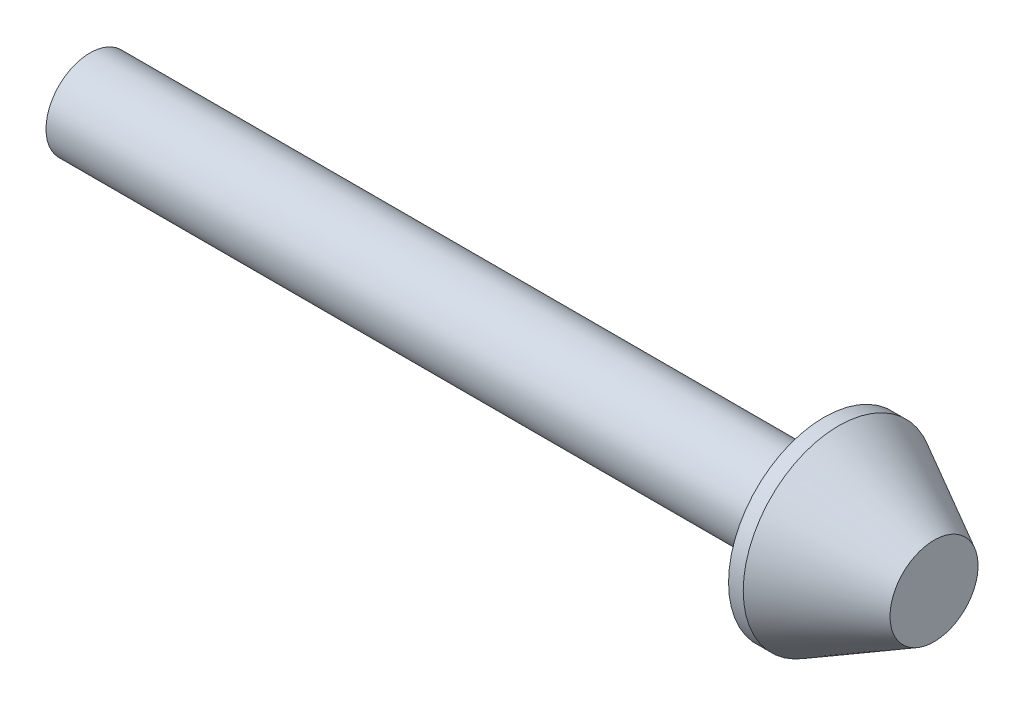
ISO-10303-21;
HEADER;
FILE_DESCRIPTION(('STEP AP214'),'2;1');
FILE_NAME('part.step','',(''),(''),'','','');
FILE_SCHEMA(('AUTOMOTIVE_DESIGN { 1 0 10303 214 1 1 1 1 }'));
ENDSEC;
DATA;
#1=APPLICATION_CONTEXT('core data for automotive mechanical design processes');
#2=APPLICATION_PROTOCOL_DEFINITION('international standard','automotive_design',2000,#1);
#3=PRODUCT_CONTEXT('',#1,'mechanical');
#4=PRODUCT('Part','Part','',(#3));
#5=PRODUCT_RELATED_PRODUCT_CATEGORY('part','',(#4));
#6=PRODUCT_DEFINITION_FORMATION('','',#4);
#7=PRODUCT_DEFINITION_CONTEXT('part definition',#1,'design');
#8=PRODUCT_DEFINITION('design','',#6,#7);
#9=PRODUCT_DEFINITION_SHAPE('','',#8);
#10=(LENGTH_UNIT() NAMED_UNIT(*) SI_UNIT(.MILLI.,.METRE.));
#11=(NAMED_UNIT(*) PLANE_ANGLE_UNIT() SI_UNIT($,.RADIAN.));
#12=(NAMED_UNIT(*) SI_UNIT($,.STERADIAN.) SOLID_ANGLE_UNIT());
#13=UNCERTAINTY_MEASURE_WITH_UNIT(LENGTH_MEASURE(1.E-05),#10,'distance_accuracy_value','');
#14=(GEOMETRIC_REPRESENTATION_CONTEXT(3) GLOBAL_UNCERTAINTY_ASSIGNED_CONTEXT((#13)) GLOBAL_UNIT_ASSIGNED_CONTEXT((#10,
#11,#12)) REPRESENTATION_CONTEXT('',''));
#15=CARTESIAN_POINT('',(0.,0.,0.));
#16=DIRECTION('',(0.,0.,1.));
#17=DIRECTION('',(1.,0.,0.));
#18=AXIS2_PLACEMENT_3D('',#15,#16,#17);
#19=CARTESIAN_POINT('',(0.,6.,0.));
#20=DIRECTION('',(1.,0.,0.));
#21=DIRECTION('',(0.,0.,-1.));
#22=AXIS2_PLACEMENT_3D('',#19,#20,#21);
#23=PLANE('',#22);
#24=CARTESIAN_POINT('',(0.,0.,0.));
#25=DIRECTION('',(-1.,0.,0.));
#26=DIRECTION('',(0.,0.,1.));
#27=AXIS2_PLACEMENT_3D('',#24,#25,#26);
#28=CIRCLE('',#27,6.);
#29=CARTESIAN_POINT('',(0.,0.,6.));
#30=VERTEX_POINT('',#29);
#31=EDGE_CURVE('E57',#30,#30,#28,.T.);
#32=ORIENTED_EDGE('',*,*,#31,.T.);
#33=EDGE_LOOP('',(#32));
#34=FACE_BOUND('',#33,.T.);
#35=ADVANCED_FACE('F40',(#34),#23,.F.);
#36=CARTESIAN_POINT('',(115.,0.,0.));
#37=DIRECTION('',(-1.,0.,0.));
#38=DIRECTION('',(0.,0.,1.));
#39=AXIS2_PLACEMENT_3D('',#36,#37,#38);
#40=PLANE('',#39);
#41=CARTESIAN_POINT('',(115.,0.,0.));
#42=DIRECTION('',(-1.,0.,0.));
#43=DIRECTION('',(0.,0.,1.));
#44=AXIS2_PLACEMENT_3D('',#41,#42,#43);
#45=CIRCLE('',#44,6.);
#46=CARTESIAN_POINT('',(115.,0.,6.));
#47=VERTEX_POINT('',#46);
#48=EDGE_CURVE('E10',#47,#47,#45,.T.);
#49=ORIENTED_EDGE('',*,*,#48,.F.);
#50=EDGE_LOOP('',(#49));
#51=FACE_BOUND('',#50,.T.);
#52=ADVANCED_FACE('F77',(#51),#40,.F.);
#53=CARTESIAN_POINT('',(115.,0.,0.));
#54=DIRECTION('',(-1.,0.,0.));
#55=DIRECTION('',(0.,0.,1.));
#56=AXIS2_PLACEMENT_3D('',#53,#54,#55);
#57=CONICAL_SURFACE('',#56,6.,0.493941368919582);
#58=CARTESIAN_POINT('',(102.,0.,0.));
#59=DIRECTION('',(-1.,0.,0.));
#60=DIRECTION('',(0.,0.,1.));
#61=AXIS2_PLACEMENT_3D('',#58,#59,#60);
#62=CIRCLE('',#61,13.);
#63=CARTESIAN_POINT('',(102.,0.,13.));
#64=VERTEX_POINT('',#63);
#65=EDGE_CURVE('E43',#64,#64,#62,.T.);
#66=ORIENTED_EDGE('',*,*,#65,.F.);
#67=EDGE_LOOP('',(#66));
#68=FACE_BOUND('',#67,.T.);
#69=ORIENTED_EDGE('',*,*,#48,.T.);
#70=EDGE_LOOP('',(#69));
#71=FACE_BOUND('',#70,.T.);
#72=ADVANCED_FACE('F73',(#68,#71),#57,.T.);
#73=CARTESIAN_POINT('',(0.,0.,0.));
#74=DIRECTION('',(-1.,0.,0.));
#75=DIRECTION('',(0.,0.,1.));
#76=AXIS2_PLACEMENT_3D('',#73,#74,#75);
#77=CYLINDRICAL_SURFACE('',#76,13.);
#78=CARTESIAN_POINT('',(100.,0.,0.));
#79=DIRECTION('',(-1.,0.,0.));
#80=DIRECTION('',(0.,0.,1.));
#81=AXIS2_PLACEMENT_3D('',#78,#79,#80);
#82=CIRCLE('',#81,13.);
#83=CARTESIAN_POINT('',(100.,0.,13.));
#84=VERTEX_POINT('',#83);
#85=EDGE_CURVE('E50',#84,#84,#82,.T.);
#86=ORIENTED_EDGE('',*,*,#85,.F.);
#87=EDGE_LOOP('',(#86));
#88=FACE_BOUND('',#87,.T.);
#89=ORIENTED_EDGE('',*,*,#65,.T.);
#90=EDGE_LOOP('',(#89));
#91=FACE_BOUND('',#90,.T.);
#92=ADVANCED_FACE('F68',(#88,#91),#77,.T.);
#93=CARTESIAN_POINT('',(100.,13.,0.));
#94=DIRECTION('',(1.,0.,0.));
#95=DIRECTION('',(0.,0.,-1.));
#96=AXIS2_PLACEMENT_3D('',#93,#94,#95);
#97=PLANE('',#96);
#98=CARTESIAN_POINT('',(100.,0.,0.));
#99=DIRECTION('',(-1.,0.,0.));
#100=DIRECTION('',(0.,0.,1.));
#101=AXIS2_PLACEMENT_3D('',#98,#99,#100);
#102=CIRCLE('',#101,6.00000000000002);
#103=CARTESIAN_POINT('',(100.,0.,6.00000000000002));
#104=VERTEX_POINT('',#103);
#105=EDGE_CURVE('E51',#104,#104,#102,.T.);
#106=ORIENTED_EDGE('',*,*,#105,.F.);
#107=EDGE_LOOP('',(#106));
#108=FACE_BOUND('',#107,.T.);
#109=ORIENTED_EDGE('',*,*,#85,.T.);
#110=EDGE_LOOP('',(#109));
#111=FACE_BOUND('',#110,.T.);
#112=ADVANCED_FACE('F63',(#108,#111),#97,.F.);
#113=CARTESIAN_POINT('',(0.,0.,0.));
#114=DIRECTION('',(-1.,0.,0.));
#115=DIRECTION('',(0.,0.,1.));
#116=AXIS2_PLACEMENT_3D('',#113,#114,#115);
#117=CYLINDRICAL_SURFACE('',#116,6.00000000000001);
#118=ORIENTED_EDGE('',*,*,#31,.F.);
#119=EDGE_LOOP('',(#118));
#120=FACE_BOUND('',#119,.T.);
#121=ORIENTED_EDGE('',*,*,#105,.T.);
#122=EDGE_LOOP('',(#121));
#123=FACE_BOUND('',#122,.T.);
#124=ADVANCED_FACE('F64',(#120,#123),#117,.T.);
#125=CLOSED_SHELL('',(#35,#52,#72,#92,#112,#124));
#126=MANIFOLD_SOLID_BREP('B2',#125);
#127=ADVANCED_BREP_SHAPE_REPRESENTATION('',(#18,#126),#14);
#128=SHAPE_DEFINITION_REPRESENTATION(#9,#127);
ENDSEC;
END-ISO-10303-21;
